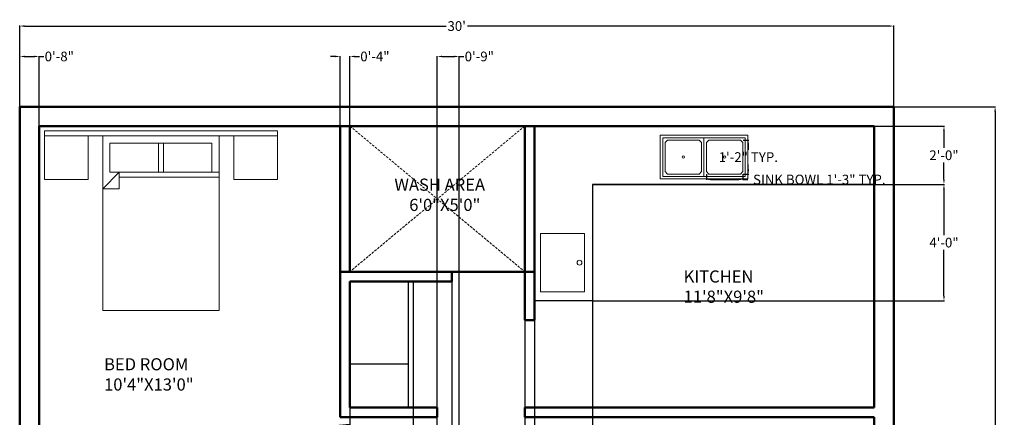
# Model space of a CAD drawing. Units: inches. Extents: x 284 to 690, y 63 to 494.
# Tile 2 of 2: x 284 to 690, y 331 to 494. Entities that reach past the tile are written whole.
import ezdxf

# ---------------------------------------------------------------- set-up
doc = ezdxf.new("R2010")
doc.units = ezdxf.units.IN
doc.header["$MEASUREMENT"] = 0
doc.linetypes.add('DASHEDX2', pattern=[1.5, 1, -0.5])
for name, color, linetype, lineweight in [('A-ANNO-DIMS', 2, 'Continuous', 18), ('A-AREA-IDEN', 7, 'Continuous', 25), ('A-DOOR', 4, 'Continuous', 25), ('A-FLOR-CASE', 32, 'Continuous', 25), ('A-FLOR-FIXT', 9, 'Continuous', 18), ('A-FURN', 8, 'Continuous', 18), ('A-ROOF-OVHD', 8, 'DASHEDX2', 18), ('A-WALL', 7, 'Continuous', 50)]:
    doc.layers.add(name, color=color, linetype=linetype, lineweight=lineweight)
doc.styles.get("Standard").update_dxf_attribs({"font": 'arial.ttf'})
doc.dimstyles.get("Standard").update_dxf_attribs({"dimtxt": 4, "dimasz": 2, "dimexe": 0.18, "dimexo": 0.0625, "dimgap": 1, "dimtad": 0, "dimtih": 1, "dimtoh": 1, "dimdec": 0, "dimzin": 0, "dimdsep": 46, "dimlunit": 3, "dimtxsty": 'Standard', "dimcen": 0.09, "dimadec": 0, "dimazin": 0, "dimtfac": 1, "dimtdec": 0, "dimtofl": 0, "dimtmove": 0, "dimatfit": 3, "dimfxl": 1, "dimtolj": 1, "dimtzin": 0, "dimarcsym": 0})

# ---------------------------------------------------------------- blocks, each defined once
blk = doc.blocks.new('*D1')
at = {"layer": 'A-ANNO-DIMS', "color": 0, "lineweight": -2, "transparency": 16777216}
for p, q in [((284.41, 458.61), (284.41, 491.96)), ((286.41, 491.78), (460.01, 491.78)), ((642.41, 491.78), (468.8, 491.78)), ((644.41, 458.61), (644.41, 491.96))]:
    blk.add_line(p, q, dxfattribs=at)
at = {"layer": 'A-ANNO-DIMS', "color": 0, "lineweight": -3, "transparency": 16777216}
for points in [[(286.41, 492.12), (286.41, 491.45), (284.41, 491.78)], [(642.41, 492.12), (642.41, 491.45), (644.41, 491.78)]]:
    blk.add_solid(points, dxfattribs=at)
at = {"layer": 'Defpoints', "color": 0, "lineweight": -3, "transparency": 16777216}
for p in [(644.41, 491.78), (284.41, 458.55), (644.41, 458.55)]:
    blk.add_point(p, dxfattribs=at)
at = {"layer": 'A-ANNO-DIMS', "color": 0, "transparency": 16777216, "insert": (464.41, 491.78), "char_height": 4, "attachment_point": 5}
blk.add_mtext("\\A1;30'", dxfattribs=at)
blk = doc.blocks.new('*D2')
at = {"layer": 'A-ANNO-DIMS', "color": 0, "lineweight": -2, "transparency": 16777216}
for p, q in [((644.47, 458.55), (686.36, 458.55)), ((686.18, 456.55), (686.18, 281.59)), ((686.18, 100.55), (686.18, 275.51)), ((644.47, 98.55), (686.36, 98.55))]:
    blk.add_line(p, q, dxfattribs=at)
at = {"layer": 'A-ANNO-DIMS', "color": 0, "lineweight": -3, "transparency": 16777216}
for points in [[(685.85, 456.55), (686.51, 456.55), (686.18, 458.55)], [(685.85, 100.55), (686.51, 100.55), (686.18, 98.55)]]:
    blk.add_solid(points, dxfattribs=at)
at = {"layer": 'Defpoints', "color": 0, "lineweight": -3, "transparency": 16777216}
for p in [(644.41, 458.55), (644.41, 98.55), (686.18, 98.55)]:
    blk.add_point(p, dxfattribs=at)
at = {"layer": 'A-ANNO-DIMS', "color": 0, "transparency": 16777216, "insert": (686.18, 278.55), "char_height": 4, "attachment_point": 5}
blk.add_mtext("\\A1;30'", dxfattribs=at)
blk = doc.blocks.new('BED-48X72')
for p, q in [((0, 0), (0, 72)), ((0, 72), (48, 72)), ((23, 69), (23, 57)), ((25, 69), (25, 57)), ((45, 69), (45, 57)), ((48, 72), (48, 0)), ((0, 50.17), (6.83, 57)), ((45, 57), (3, 57)), ((6.83, 57), (6.83, 50.17)), ((45, 57), (48, 57)), ((48, 57), (48, 54)), ((48, 55), (6.83, 55)), ((0, 50.17), (6.83, 50.17)), ((48, 0), (0, 0))]:
    blk.add_line(p, q)
blk.add_lwpolyline([(3, 57), (3, 69), (45, 69), (45, 57)])
blk = doc.blocks.new('DOOR-SINGLE-30')
for p, q in [((30, 33), (0, 33)), ((0, 33), (0, 32)), ((30, 36), (30, 33)), ((30, 33), (30, 32)), ((0, 32), (30, 32)), ((30, 0), (30, 3))]:
    blk.add_line(p, q)
blk.add_arc((29.02, 32), 29.02, 180, 271.942)
blk = doc.blocks.new('SINK-BOWL-15X14')
for p, q in [((0, 13), (1, 14)), ((0, 1), (0, 13)), ((1, 14), (14, 14)), ((14, 14), (15, 13)), ((15, 13), (15, 1)), ((0, 1), (1, 0)), ((15, 1), (14, 0)), ((14, 0), (1, 0))]:
    blk.add_line(p, q)
blk.add_circle((7.5, 7), 0.5)
blk = doc.blocks.new('TABLE-SIDE-18SQ')
blk.add_lwpolyline([(18, 18), (18, 0), (0, 0), (0, 18)], close=True)
blk = doc.blocks.new('*D13')
at = {"layer": 'A-ANNO-DIMS', "color": 0, "lineweight": -2, "transparency": 16777216}
for p, q in [((567.27, 430.73), (567.27, 428.36)), ((582.27, 430.73), (582.27, 428.36)), ((569.27, 428.54), (580.27, 428.54)), ((582.27, 428.54), (584.27, 428.54))]:
    blk.add_line(p, q, dxfattribs=at)
at = {"layer": 'A-ANNO-DIMS', "color": 0, "lineweight": -3, "transparency": 16777216}
for points in [[(569.27, 428.87), (569.27, 428.21), (567.27, 428.54)], [(580.27, 428.87), (580.27, 428.21), (582.27, 428.54)]]:
    blk.add_solid(points, dxfattribs=at)
at = {"layer": 'Defpoints', "color": 0, "lineweight": -3, "transparency": 16777216}
for p in [(567.27, 430.79), (582.27, 430.79), (582.27, 428.54)]:
    blk.add_point(p, dxfattribs=at)
at = {"layer": 'A-ANNO-DIMS', "color": 0, "transparency": 16777216, "insert": (613.76, 428.54), "char_height": 4, "attachment_point": 5}
blk.add_mtext('\\A1;SINK BOWL 1\'-3" TYP.', dxfattribs=at)
blk = doc.blocks.new('*D14')
at = {"layer": 'A-ANNO-DIMS', "color": 0, "lineweight": -2, "transparency": 16777216}
for p, q in [((582.34, 444.79), (584.7, 444.79)), ((584.52, 442.79), (584.52, 440.8)), ((584.52, 432.79), (584.52, 434.78)), ((582.34, 430.79), (584.7, 430.79))]:
    blk.add_line(p, q, dxfattribs=at)
at = {"layer": 'A-ANNO-DIMS', "color": 0, "lineweight": -3, "transparency": 16777216}
for points in [[(584.19, 442.79), (584.86, 442.79), (584.52, 444.79)], [(584.19, 432.79), (584.86, 432.79), (584.52, 430.79)]]:
    blk.add_solid(points, dxfattribs=at)
at = {"layer": 'Defpoints', "color": 0, "lineweight": -3, "transparency": 16777216}
for p in [(582.27, 444.79), (584.52, 444.79), (582.27, 430.79)]:
    blk.add_point(p, dxfattribs=at)
at = {"layer": 'A-ANNO-DIMS', "color": 0, "transparency": 16777216, "insert": (584.52, 437.79), "char_height": 4, "attachment_point": 5}
blk.add_mtext('\\A1;1\'-2" TYP.', dxfattribs=at)
blk = doc.blocks.new('*D23')
at = {"layer": 'A-ANNO-DIMS', "color": 0, "lineweight": -2, "transparency": 16777216}
for p, q in [((284.41, 458.61), (284.41, 479.43)), ((286.41, 479.25), (290.41, 479.25)), ((292.41, 450.61), (292.41, 479.43)), ((292.41, 479.25), (294.41, 479.25))]:
    blk.add_line(p, q, dxfattribs=at)
at = {"layer": 'A-ANNO-DIMS', "color": 0, "lineweight": -3, "transparency": 16777216}
for points in [[(286.41, 479.58), (286.41, 478.92), (284.41, 479.25)], [(290.41, 479.58), (290.41, 478.92), (292.41, 479.25)]]:
    blk.add_solid(points, dxfattribs=at)
at = {"layer": 'Defpoints', "color": 0, "lineweight": -3, "transparency": 16777216}
for p in [(292.41, 479.25), (284.41, 458.55), (292.41, 450.55)]:
    blk.add_point(p, dxfattribs=at)
at = {"layer": 'A-ANNO-DIMS', "color": 0, "transparency": 16777216, "insert": (300.72, 479.25), "char_height": 4, "attachment_point": 5}
blk.add_mtext('\\A1;0\'-8"', dxfattribs=at)
blk = doc.blocks.new('*D24')
at = {"layer": 'A-ANNO-DIMS', "color": 0, "lineweight": -2, "transparency": 16777216}
for p, q in [((414.41, 479.25), (412.41, 479.25)), ((416.41, 450.61), (416.41, 479.43)), ((420.41, 450.61), (420.41, 479.43)), ((422.41, 479.25), (424.41, 479.25))]:
    blk.add_line(p, q, dxfattribs=at)
at = {"layer": 'A-ANNO-DIMS', "color": 0, "lineweight": -3, "transparency": 16777216}
for points in [[(414.41, 479.58), (414.41, 478.92), (416.41, 479.25)], [(422.41, 479.58), (422.41, 478.92), (420.41, 479.25)]]:
    blk.add_solid(points, dxfattribs=at)
at = {"layer": 'Defpoints', "color": 0, "lineweight": -3, "transparency": 16777216}
for p in [(420.41, 479.25), (416.41, 450.55), (420.41, 450.55)]:
    blk.add_point(p, dxfattribs=at)
at = {"layer": 'A-ANNO-DIMS', "color": 0, "transparency": 16777216, "insert": (430.72, 479.25), "char_height": 4, "attachment_point": 5}
blk.add_mtext('\\A1;0\'-4"', dxfattribs=at)
blk = doc.blocks.new('*D27')
at = {"layer": 'A-ANNO-DIMS', "color": 0, "lineweight": -2, "transparency": 16777216}
for p, q in [((456.41, 178.61), (456.41, 479.43)), ((458.41, 479.25), (463.41, 479.25)), ((465.41, 178.61), (465.41, 479.43)), ((465.41, 479.25), (467.41, 479.25))]:
    blk.add_line(p, q, dxfattribs=at)
at = {"layer": 'A-ANNO-DIMS', "color": 0, "lineweight": -3, "transparency": 16777216}
for points in [[(458.41, 479.58), (458.41, 478.92), (456.41, 479.25)], [(463.41, 479.58), (463.41, 478.92), (465.41, 479.25)]]:
    blk.add_solid(points, dxfattribs=at)
at = {"layer": 'Defpoints', "color": 0, "lineweight": -3, "transparency": 16777216}
for p in [(465.41, 479.25), (456.41, 178.55), (465.41, 178.55)]:
    blk.add_point(p, dxfattribs=at)
at = {"layer": 'A-ANNO-DIMS', "color": 0, "transparency": 16777216, "insert": (473.72, 479.25), "char_height": 4, "attachment_point": 5}
blk.add_mtext('\\A1;0\'-9"', dxfattribs=at)
blk = doc.blocks.new('*D29')
at = {"layer": 'A-ANNO-DIMS', "color": 0, "lineweight": -2, "transparency": 16777216}
for p, q in [((636.47, 450.55), (665.29, 450.55)), ((665.11, 448.55), (665.11, 441.59)), ((665.11, 428.55), (665.11, 435.51)), ((636.47, 426.55), (665.29, 426.55))]:
    blk.add_line(p, q, dxfattribs=at)
at = {"layer": 'A-ANNO-DIMS', "color": 0, "lineweight": -3, "transparency": 16777216}
for points in [[(664.77, 448.55), (665.44, 448.55), (665.11, 450.55)], [(664.77, 428.55), (665.44, 428.55), (665.11, 426.55)]]:
    blk.add_solid(points, dxfattribs=at)
at = {"layer": 'Defpoints', "color": 0, "lineweight": -3, "transparency": 16777216}
for p in [(636.41, 450.55), (636.41, 426.55), (665.11, 426.55)]:
    blk.add_point(p, dxfattribs=at)
at = {"layer": 'A-ANNO-DIMS', "color": 0, "transparency": 16777216, "insert": (665.11, 438.55), "char_height": 4, "attachment_point": 5}
blk.add_mtext('\\A1;2\'-0"', dxfattribs=at)
blk = doc.blocks.new('*D30')
at = {"layer": 'A-ANNO-DIMS', "color": 0, "lineweight": -2, "transparency": 16777216}
for p, q in [((496.41, 378.49), (496.41, 65.67)), ((520.41, 378.49), (520.41, 65.67)), ((498.41, 65.85), (502.06, 65.85)), ((518.41, 65.85), (514.76, 65.85))]:
    blk.add_line(p, q, dxfattribs=at)
at = {"layer": 'A-ANNO-DIMS', "color": 0, "lineweight": -3, "transparency": 16777216}
for points in [[(498.41, 66.18), (498.41, 65.52), (496.41, 65.85)], [(518.41, 66.18), (518.41, 65.52), (520.41, 65.85)]]:
    blk.add_solid(points, dxfattribs=at)
at = {"layer": 'Defpoints', "color": 0, "lineweight": -3, "transparency": 16777216}
for p in [(496.41, 378.55), (520.41, 378.55), (520.41, 65.85)]:
    blk.add_point(p, dxfattribs=at)
at = {"layer": 'A-ANNO-DIMS', "color": 0, "transparency": 16777216, "insert": (508.41, 65.85), "char_height": 4, "attachment_point": 5}
blk.add_mtext('\\A1;2\'-0"', dxfattribs=at)
blk = doc.blocks.new('*D31')
at = {"layer": 'A-ANNO-DIMS', "color": 0, "lineweight": -2, "transparency": 16777216}
for p, q in [((520.47, 426.55), (665.29, 426.55)), ((665.11, 424.55), (665.11, 405.59)), ((665.11, 380.55), (665.11, 399.51)), ((520.47, 378.55), (665.29, 378.55))]:
    blk.add_line(p, q, dxfattribs=at)
at = {"layer": 'A-ANNO-DIMS', "color": 0, "lineweight": -3, "transparency": 16777216}
for points in [[(664.77, 424.55), (665.44, 424.55), (665.11, 426.55)], [(664.77, 380.55), (665.44, 380.55), (665.11, 378.55)]]:
    blk.add_solid(points, dxfattribs=at)
at = {"layer": 'Defpoints', "color": 0, "lineweight": -3, "transparency": 16777216}
for p in [(520.41, 426.55), (665.11, 426.55), (520.41, 378.55)]:
    blk.add_point(p, dxfattribs=at)
at = {"layer": 'A-ANNO-DIMS', "color": 0, "transparency": 16777216, "insert": (665.11, 402.55), "char_height": 4, "attachment_point": 5}
blk.add_mtext('\\A1;4\'-0"', dxfattribs=at)
blk = doc.blocks.new('*D32')
at = {"layer": 'A-ANNO-DIMS', "color": 0, "lineweight": -2, "transparency": 16777216}
for p, q in [((492.41, 390.49), (492.41, 65.67)), ((462.41, 386.49), (462.41, 65.67)), ((464.41, 65.85), (471.06, 65.85)), ((490.41, 65.85), (483.76, 65.85))]:
    blk.add_line(p, q, dxfattribs=at)
at = {"layer": 'A-ANNO-DIMS', "color": 0, "lineweight": -3, "transparency": 16777216}
for points in [[(464.41, 66.18), (464.41, 65.52), (462.41, 65.85)], [(490.41, 66.18), (490.41, 65.52), (492.41, 65.85)]]:
    blk.add_solid(points, dxfattribs=at)
at = {"layer": 'Defpoints', "color": 0, "lineweight": -3, "transparency": 16777216}
for p in [(492.41, 390.55), (462.41, 386.55), (492.41, 65.85)]:
    blk.add_point(p, dxfattribs=at)
at = {"layer": 'A-ANNO-DIMS', "color": 0, "transparency": 16777216, "insert": (477.41, 65.85), "char_height": 4, "attachment_point": 5}
blk.add_mtext('\\A1;2\'-6"', dxfattribs=at)
blk = doc.blocks.new('*D33')
at = {"layer": 'A-ANNO-DIMS', "color": 0, "lineweight": -2, "transparency": 16777216}
for p, q in [((420.41, 334.49), (420.41, 65.67)), ((446.41, 334.49), (446.41, 65.67)), ((422.41, 65.85), (427.06, 65.85)), ((444.41, 65.85), (439.76, 65.85))]:
    blk.add_line(p, q, dxfattribs=at)
at = {"layer": 'A-ANNO-DIMS', "color": 0, "lineweight": -3, "transparency": 16777216}
for points in [[(422.41, 66.18), (422.41, 65.52), (420.41, 65.85)], [(444.41, 66.18), (444.41, 65.52), (446.41, 65.85)]]:
    blk.add_solid(points, dxfattribs=at)
at = {"layer": 'Defpoints', "color": 0, "lineweight": -3, "transparency": 16777216}
for p in [(420.41, 334.55), (446.41, 334.55), (446.41, 65.85)]:
    blk.add_point(p, dxfattribs=at)
at = {"layer": 'A-ANNO-DIMS', "color": 0, "transparency": 16777216, "insert": (433.41, 65.85), "char_height": 4, "attachment_point": 5}
blk.add_mtext('\\A1;2\'-2"', dxfattribs=at)

msp = doc.modelspace()

# ---------------------------------------------------------------- linework, layer by layer
at = {"layer": 'A-FLOR-CASE'}
for p, q in [((636.41, 450.55), (636.41, 426.55)), ((636.41, 426.55), (520.41, 426.55)), ((520.41, 426.55), (520.41, 378.55)), ((444.41, 386.55), (444.41, 334.55)), ((446.41, 386.55), (446.41, 334.55)), ((520.41, 378.55), (496.41, 378.55)), ((420.41, 352.55), (444.41, 352.55))]:
    msp.add_line(p, q, dxfattribs=at)
at = {"layer": 'A-FLOR-FIXT'}
for p, q in [((548.27, 446.79), (584.27, 446.79)), ((548.27, 428.79), (548.27, 446.79)), ((584.27, 446.79), (584.27, 428.79)), ((549.27, 445.79), (583.27, 445.79)), ((549.27, 429.79), (549.27, 445.79)), ((566.27, 445.79), (566.27, 429.79)), ((583.27, 445.79), (583.27, 429.79)), ((584.27, 428.79), (548.27, 428.79)), ((583.27, 429.79), (549.27, 429.79))]:
    msp.add_line(p, q, dxfattribs=at)
msp.add_lwpolyline([(498.98, 406.27), (516.98, 406.27), (516.98, 382.27), (498.98, 382.27)], close=True, dxfattribs=at)
msp.add_circle((514.98, 394.27), 1, dxfattribs=at)
at = {"layer": 'A-FURN'}
for p, q in [((292.41, 450.55), (292.41, 448.55)), ((294.6, 448.55), (390.6, 448.55)), ((294.6, 446.55), (294.6, 448.55)), ((390.6, 446.55), (294.6, 446.55)), ((390.6, 446.55), (390.6, 448.55)), ((416.41, 448.55), (416.41, 446.55))]:
    msp.add_line(p, q, dxfattribs=at)
at = {"layer": 'A-ROOF-OVHD'}
for p, q in [((420.41, 450.55), (492.41, 390.55)), ((492.41, 450.55), (420.41, 390.55))]:
    msp.add_line(p, q, dxfattribs=at)
at = {"layer": 'A-WALL'}
for p, q in [((284.41, 458.55), (644.41, 458.55)), ((284.41, 98.55), (284.41, 458.55)), ((644.41, 458.55), (644.41, 98.55)), ((292.41, 450.55), (636.41, 450.55)), ((292.41, 242.55), (292.41, 450.55)), ((416.41, 330.55), (416.41, 450.55)), ((420.41, 390.55), (420.41, 450.55)), ((492.41, 370.55), (492.41, 450.55)), ((496.41, 370.55), (496.41, 450.55)), ((636.41, 334.55), (636.41, 450.55)), ((416.41, 390.55), (462.41, 390.55)), ((462.41, 390.55), (462.41, 386.55)), ((462.41, 390.55), (492.41, 390.55)), ((492.41, 390.55), (496.41, 390.55)), ((420.41, 386.55), (462.41, 386.55)), ((420.41, 334.55), (420.41, 386.55)), ((492.41, 370.55), (496.41, 370.55)), ((420.41, 334.55), (456.41, 334.55)), ((456.41, 334.55), (456.41, 330.55)), ((492.41, 330.55), (492.41, 334.55)), ((492.41, 334.55), (492.41, 330.55)), ((492.41, 334.55), (636.41, 334.55)), ((416.41, 330.55), (456.41, 330.55)), ((420.41, 330.55), (444.41, 330.55)), ((492.41, 330.55), (496.41, 330.55)), ((492.41, 330.55), (636.41, 330.55)), ((636.41, 98.55), (636.41, 330.55))]:
    msp.add_line(p, q, dxfattribs=at)

# ---------------------------------------------------------------- block references
at = {"layer": 'A-DOOR', "extrusion": (0, 0, -1), "zscale": -1, "rotation": 180}
msp.add_blockref('DOOR-SINGLE-30', (-390.41, 330.55), dxfattribs=at)
at = {"layer": 'A-FLOR-FIXT'}
for p in [(550.27, 430.79), (567.27, 430.79)]:
    msp.add_blockref('SINK-BOWL-15X14', p, dxfattribs=at)
at = {"layer": 'A-FURN'}
for name, p in [('TABLE-SIDE-18SQ', (294.6, 428.55)), ('BED-48X72', (318.6, 374.55)), ('TABLE-SIDE-18SQ', (372.6, 428.55))]:
    msp.add_blockref(name, p, dxfattribs=at)

# ---------------------------------------------------------------- texts
at = {"layer": 'A-AREA-IDEN', "char_height": 5, "attachment_point": 1}
for s, insert in [('WASH AREA\\P    6\'0"X5\'0"', (438.74, 428.92)), ('KITCHEN\\P11\'8"X9\'8"', (557.88, 391.08)), ('BED ROOM\\P10\'4"X13\'0"', (319.16, 354.91))]:
    msp.add_mtext_dynamic_manual_height_columns(s, width=85.9248, gutter_width=1, heights=[0], dxfattribs=dict(at, insert=insert))

# ---------------------------------------------------------------- dimensions: what is measured, and where the dimension line sits
at = {"layer": 'A-ANNO-DIMS'}
for base, p1, p2, override, picture, middle in [((644.41, 491.78), (284.41, 458.55), (644.41, 458.55), {"dimclrd": 0, "dimclre": 0, "dimclrt": 0}, '*D1', (464.41, 491.78)), ((292.41, 479.25), (284.41, 458.55), (292.41, 450.55), {"dimdec": 1, "dimlfac": 1, "dimrnd": 0, "dimzin": 1, "dimdsep": 46, "dimlunit": 4, "dimfrac": 2}, '*D23', (300.72, 479.25)), ((420.41, 479.25), (416.41, 450.55), (420.41, 450.55), {"dimdec": 1, "dimlfac": 1, "dimrnd": 0, "dimzin": 1, "dimdsep": 46, "dimlunit": 4, "dimfrac": 2}, '*D24', (430.72, 479.25)), ((465.41, 479.25), (456.41, 178.55), (465.41, 178.55), {"dimdec": 1, "dimlfac": 1, "dimrnd": 0, "dimzin": 1, "dimdsep": 46, "dimlunit": 4, "dimfrac": 2}, '*D27', (473.72, 479.25)), ((492.41, 65.85), (462.41, 386.55), (492.41, 390.55), {"dimdec": 1, "dimlfac": 1, "dimrnd": 0, "dimzin": 1, "dimdsep": 46, "dimlunit": 4, "dimfrac": 2}, '*D32', (477.41, 65.85)), ((520.41, 65.85), (496.41, 378.55), (520.41, 378.55), {"dimdec": 1, "dimlfac": 1, "dimrnd": 0, "dimzin": 1, "dimdsep": 46, "dimlunit": 4, "dimfrac": 2}, '*D30', (508.41, 65.85)), ((446.41, 65.85), (420.41, 334.55), (446.41, 334.55), {"dimdec": 1, "dimlfac": 1, "dimrnd": 0, "dimzin": 1, "dimdsep": 46, "dimlunit": 4, "dimfrac": 2}, '*D33', (433.41, 65.85))]:
    dim = msp.add_linear_dim(base=base, p1=p1, p2=p2, dimstyle='Standard', override=override, dxfattribs=at)
    dim.commit()
    dim.dimension.update_dxf_attribs({"geometry": picture, "text_midpoint": middle})
for base, p1, p2, override, picture, middle in [((686.18, 98.55), (644.41, 458.55), (644.41, 98.55), {"dimclrd": 0, "dimclre": 0, "dimclrt": 0}, '*D2', (686.18, 278.55)), ((665.11, 426.55), (636.41, 450.55), (636.41, 426.55), {"dimdec": 1, "dimlfac": 1, "dimrnd": 0, "dimzin": 1, "dimdsep": 46, "dimlunit": 4, "dimfrac": 2}, '*D29', (665.11, 438.55)), ((665.11, 426.55), (520.41, 378.55), (520.41, 426.55), {"dimdec": 1, "dimlfac": 1, "dimrnd": 0, "dimzin": 1, "dimdsep": 46, "dimlunit": 4, "dimfrac": 2}, '*D31', (665.11, 402.55))]:
    dim = msp.add_linear_dim(base=base, p1=p1, p2=p2, angle=90, dimstyle='Standard', override=override, dxfattribs=at)
    dim.commit()
    dim.dimension.update_dxf_attribs({"geometry": picture, "text_midpoint": middle})
dim = msp.add_linear_dim(base=(584.52, 444.79), p1=(582.27, 430.79), p2=(582.27, 444.79), angle=90, text='<> TYP.', dimstyle='Standard', override={"dimdec": 1, "dimlfac": 1, "dimrnd": 0, "dimzin": 1, "dimdsep": 46, "dimlunit": 4, "dimfrac": 2}, dxfattribs=at)
dim.commit()
dim.dimension.update_dxf_attribs({"geometry": '*D14', "text_midpoint": (584.52, 437.79)})
dim = msp.add_linear_dim(base=(582.27, 428.54), p1=(567.27, 430.79), p2=(582.27, 430.79), text='SINK BOWL <> TYP.', dimstyle='Standard', override={"dimdec": 1, "dimlfac": 1, "dimrnd": 0, "dimzin": 1, "dimdsep": 46, "dimlunit": 4, "dimfrac": 2}, dxfattribs=at)
dim.commit()
dim.dimension.update_dxf_attribs({"geometry": '*D13', "text_midpoint": (613.76, 428.54)})

doc.saveas('drawing.dxf')
